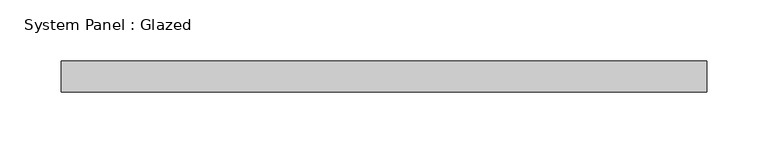
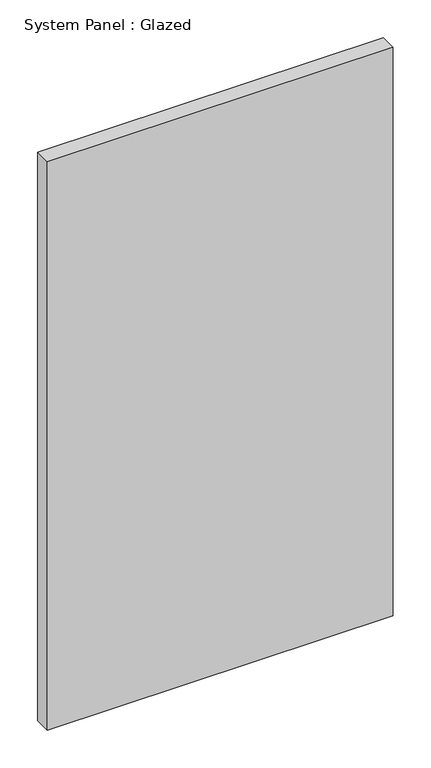
"""IFC4 building model written with IfcOpenShell, lengths in millimetres: plate geometry, System Panel : Glazed."""

from ifc_helpers import new_model, si_unit, origin, origin_with_axes, place, context, project, spatial, polyline, outline, extrude, source, transform, mapped, element, save


def system_panel_glazed_9e372a4a(model_context):
    return source(origin(), model_context, "Body", "SweptSolid", [
        extrude(outline(polyline([(264.5833333, 19.05), (-264.5833333, 19.05), (-264.5833333, 44.45), (264.5833333, 44.45), (264.5833333, 19.05)])), origin_with_axes(), (0.0, 0.0, 1.0), 918.6175922),
    ])


if __name__ == "__main__":
    model = new_model("IFC4")
    model_context = context("Model", 3, world=origin())
    ifc_project = project(units=[si_unit("LENGTHUNIT", "METRE", prefix="MILLI")], contexts=[model_context])
    site = spatial("IfcSite", under=ifc_project)
    building = spatial("IfcBuilding", under=site)
    placement = place(None, origin())
    system_panel_glazed_shape = system_panel_glazed_9e372a4a(model_context)
    element("IfcPlate", 1, ObjectType="System Panel : Glazed", at=placement, inside=building, context=model_context, shape_type="MappedRepresentation", body=[
        mapped(system_panel_glazed_shape, transform((0.0, 0.0, 0.0), x_axis=(1.0, 0.0, 0.0), y_axis=(0.0, 1.0, 0.0), z_axis=(0.0, 0.0, 1.0))),
    ])
    save(model, "model.ifc")

# Revit data of these elements
# Type "System Panel : Glazed"
#   Construction Type Id = "GSP4R"
#   Analytic Construction = "1/8 in Pilkington single glazing"
#   Visual Light Transmittance = 0.9
#   Solar Heat Gain Coefficient = 0.86
#   Heat Transfer Coefficient (U) = 1.18115 BTU/(h·ft²·°F)
#   Define Thermal Properties by = 1
# Element 1 (IfcPlate, "System Panel : Glazed")
#   Materials on its faces: "Glass"
# Materials
#   "Glass": class "Glass", colour RGB 0 128 192, transparency 0.75, Description = "Soda Lime Glass", Cost = 0
